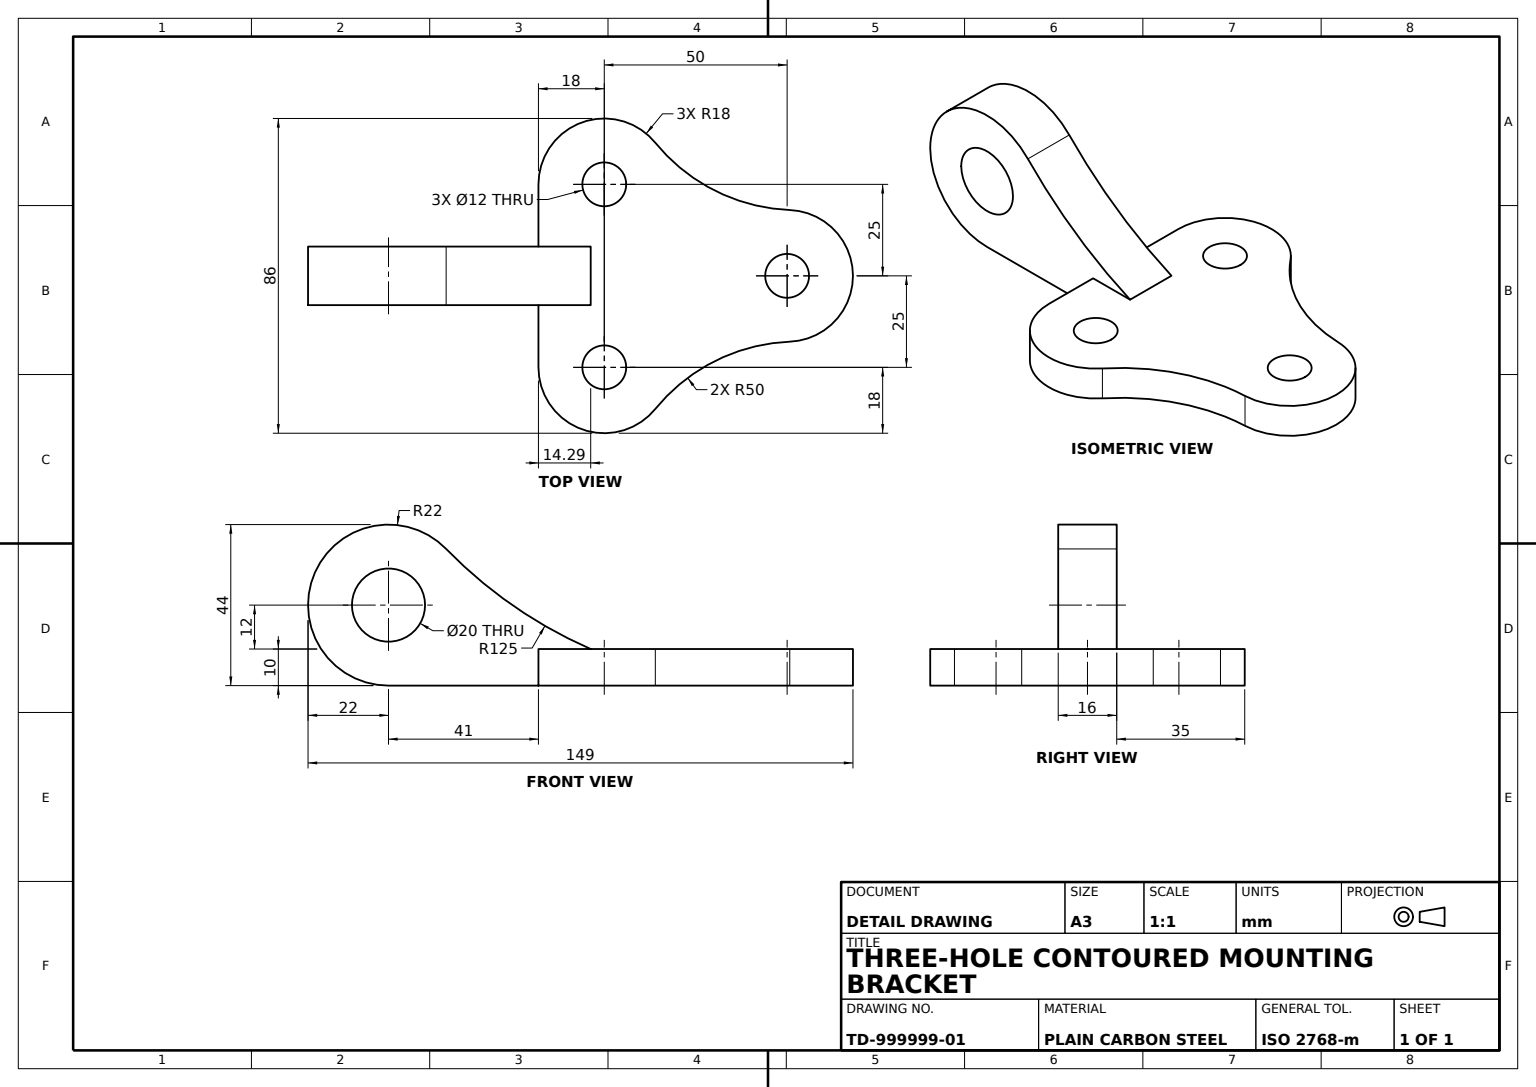
SolidWorks part; units mm, degrees
material "Plain Carbon Steel"
ref_plane "Front Plane" through (0, 0, 0) normal (0, 0, 1) x (1, 0, 0)
ref_plane "Top Plane" through (0, 0, 0) normal (0, 1, 0) x (1, 0, 0)
ref_plane "Right Plane" through (0, 0, 0) normal (1, 0, 0) x (0, 0, -1)
sketch "Base Plate Sketch" plane through (0, 0, 0) normal (0, 1, 0) x (1, 0, 0)
  line L0 (25, -68) -> (8, -68)
  line L1 (-8, -68) -> (-25, -68)
  line L3 (-8, -68) -> (-8, -53.71)
  line L4 (-8, -53.71) -> (8, -53.71)
  line L5 (8, -68) -> (8, -53.71)
  arc A0 (17.9856, 0.7207) -> (-17.9856, 0.7207) centre (0, 0) ccw
  circle A1 centre (0, 0) radius 6
  arc A2 (-36.3679, -36.044) -> (-25, -68) centre (-25, -50) ccw
  circle A3 centre (-25, -50) radius 6
  circle A4 centre (25, -50) radius 6
  arc A5 (25, -68) -> (36.3679, -36.044) centre (25, -50) ccw
  arc A6 (17.9856, 0.7207) -> (36.3679, -36.044) centre (67.9455, 2.7227) ccw
  arc A7 (-17.9856, 0.7207) -> (-36.3679, -36.044) centre (-67.9455, 2.7227) cw
  dimension "D1" = 36
  dimension "D2" = 12
  dimension "D3" = 36
  dimension "D4" = 12
  dimension "D5" = 36
  dimension "D6" = 12
  dimension "D11" = 50
  dimension "D12" = 50
  dimension "D7" = 25
  dimension "D8" = 14.29
  dimension "D9" = 50
  dimension "D10" = 25
  dimension "D13" = 8
  dimension "D14" = 16
extrude "Base Plate" add sketch "Base Plate Sketch" along normal blind 10
ref_plane "Pivot Lug Plane" through (0, 0, 0) normal (1, 0, 0) x (0, 0, -1)
sketch "Pivot Lug Sketch" plane through (0, 0, 0) normal (1, 0, 0) x (0, 0, -1)
  line L0 (-109, 0) -> (-53.71, 0)
  line L1 (-53.71, 10) -> (-53.71, 0)
  arc A0 (-93.2379, 37.3479) -> (-109, 0) centre (-109, 22) ccw
  circle A1 centre (-109, 22) radius 10
  arc A2 (-93.2379, 37.3479) -> (-53.71, 10) centre (-3.6806, 124.5515) ccw
  dimension "D1" = 44
  dimension "D2" = 20
  dimension "D5" = 125
  dimension "D3" = 22
  dimension "D4" = 41
extrude "Pivot Lug" add sketch "Pivot Lug Sketch" along normal mid plane 16
